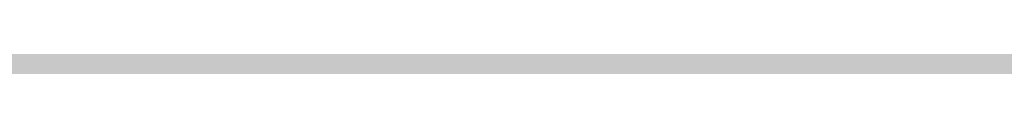
# Model space of a CAD drawing. Units: inches. Extents: x 2091 to 2899, y 967 to 2217.
# Tile 226 of 256: x 2203.4104 to 2203.7172, y 1152.2487 to 1152.2504. Entities that reach past the tile are written whole.
import ezdxf

# ---------------------------------------------------------------- set-up
doc = ezdxf.new("R2010")
doc.units = ezdxf.units.IN
doc.layers.add('A-WALL-PATT', color=141, linetype='Continuous', lineweight=13, true_color=0xadddf7)

msp = doc.modelspace()

# ---------------------------------------------------------------- hatches: boundary and pattern name
at = {"layer": 'A-WALL-PATT'}
h = msp.add_hatch(color=256, dxfattribs=at)
h.dxf.hatch_style = 1
h.paths.add_polyline_path([(2803.1436, 2050.91906), (2203.1436, 2050.91906), (2203.1436, 1090.91906), (2803.1436, 1090.91906)])
h.paths.add_polyline_path([(2635.79885, 1147.54046), (2674.52405, 1147.54046, 0.376086), (2678.52967, 1152.8802), (2678.52967, 1159.55647, 0.333335), (2674.52432, 1163.56185), (2674.52432, 1163.56185), (2674.52432, 1192.93439), (2635.80597, 1192.93439), (2597.08762, 1192.93439), (2597.08762, 1163.56185, 0.333335), (2593.08228, 1159.55647), (2593.08228, 1152.8802, 0.376086), (2597.08789, 1147.54046)], flags=0)
h.paths.add_polyline_path([(2436.01043, 1278.24078, 0.000483), (2435.95264, 1278.21503, -0.001328), (2435.93563, 1278.11169, -0.001711), (2436.11644, 1278.04076, 0.002185)], flags=0)
h.paths.add_polyline_path([(2794.1436, 1143.41906), (2794.1436, 1347.41906), (2543.37017, 1347.41906), (2543.37017, 1351.91906), (2794.1436, 1351.91906), (2794.1436, 1392.71355), (2793.9474, 1392.71355), (2793.9474, 1473.5369), (2794.1436, 1473.5369), (2794.1436, 1531.91906), (2650.1436, 1531.91906), (2650.1436, 1536.41906), (2794.1436, 1536.41906), (2794.1436, 1692.41906), (2609.37561, 1692.41906), (2609.37561, 1644.41906), (2604.87561, 1644.41906), (2604.87561, 1744.91906), (2609.37561, 1744.91906), (2609.37561, 1696.91906), (2794.1436, 1696.91906), (2794.1436, 1780.91906), (2609.6436, 1780.91906), (2493.87561, 1780.91906), (2493.87561, 1785.41906), (2609.6436, 1785.41906), (2794.1436, 1785.41906), (2794.1436, 1847.93882), (2793.95122, 1847.93882), (2793.95122, 1928.76217), (2794.1436, 1928.76217), (2794.1436, 1941.41906), (2614.1436, 1941.41906), (2614.1436, 1821.41906), (2609.6436, 1821.41906), (2609.6436, 1941.41906), (2392.1436, 1941.41906), (2392.1436, 1819.91906), (2387.6436, 1819.91906), (2387.6436, 1941.41906), (2212.1436, 1941.41906), (2212.1436, 1783.91906), (2392.1436, 1783.91906), (2392.1436, 1780.91906), (2212.1436, 1780.91906), (2212.1436, 1629.41906), (2387.6436, 1629.41906), (2387.6436, 1744.91906), (2392.1436, 1744.91906), (2392.1436, 1627.91906), (2317.1436, 1627.91906), (2317.1436, 1551.41906), (2317.1436, 1536.41906), (2459.38359, 1536.41906), (2459.38359, 1602.39648), (2463.88359, 1602.39648), (2463.88359, 1531.91906), (2456.6436, 1531.91906), (2456.6436, 1529.91906), (2452.1436, 1529.91906), (2452.1436, 1531.91906), (2312.6436, 1531.91906), (2312.6436, 1551.41906), (2306.1436, 1551.41906), (2306.1436, 1555.91906), (2308.1436, 1555.91906), (2308.1436, 1551.41906), (2312.6436, 1551.41906), (2312.6436, 1627.91906), (2212.1436, 1627.91906), (2212.1436, 1555.91906), (2270.1436, 1555.91906), (2270.1436, 1551.41906), (2212.1436, 1551.41906), (2212.1436, 1351.91906), (2272.1436, 1351.91906), (2272.1436, 1347.41906), (2212.1436, 1347.41906), (2212.1436, 1275.41906), (2308.1436, 1275.41906), (2308.1436, 1351.91906), (2452.1436, 1351.91906), (2452.1436, 1493.91906), (2456.6436, 1493.91906), (2456.6436, 1347.41906), (2312.6436, 1347.41906), (2312.6436, 1270.91906), (2212.1436, 1270.91906), (2212.1436, 1099.91906), (2281.23752, 1099.91906), (2282.87104, 1110.9138), (2282.00834, 1116.9966), (2278.55774, 1121.4204), (2268.20564, 1128.0562), (2272.08764, 1128.0562), (2273.81294, 1131.927), (2279.42034, 1134.6919), (2285.02784, 1135.2449), (2287.61584, 1137.4568), (2288.04714, 1138.0098), (2289.34114, 1140.7747), (2291.06654, 1139.6687), (2292.36054, 1135.2449), (2295.37984, 1136.9038), (2296.24254, 1135.7979), (2297.10524, 1133.033), (2300.12464, 1138.0098), (2303.14394, 1138.0098), (2304.43794, 1135.7979), (2303.14394, 1133.586), (2306.59464, 1134.6919), (2307.88874, 1133.033), (2310.90804, 1135.2449), (2313.92744, 1134.1389), (2315.62686, 1132.4271), (2308.32004, 1117.5496), (2290.20384, 1109.8079), (2288.90984, 1103.1721), (2289.27231, 1099.91906), (2434.91823, 1099.91906), (2431.59323, 1124.78806), (2429.93023, 1169.55306), (2430.92718, 1240.51969), (2435.65893, 1238.18613), (2437.13523, 1196.55406), (2438.79823, 1143.97306), (2442.67823, 1111.99806), (2446.55823, 1099.91906), (2794.1436, 1099.91906), (2794.1436, 1138.91906), (2548.03245, 1138.91906), (2548.03245, 1143.41906), (2548.03245, 1148.81906), (2546.66846, 1148.03156), (2528.68569, 1179.17862, 0.256256), (2512.03245, 1148.81906), (2512.03245, 1143.41906), (2512.03245, 1138.91906), (2507.53245, 1138.91906), (2507.53245, 1143.41906), (2507.53245, 1148.81906, 0.256256), (2490.8792, 1179.17862), (2472.89644, 1148.03156), (2471.53245, 1148.81906), (2471.53245, 1143.41906), (2467.03245, 1143.41906), (2467.03245, 1269.94579, 0.039061), (2460.90999, 1273.58006), (2467.03245, 1273.58006), (2467.03245, 1286.32536, 0.014511), (2465.21619, 1286.76191), (2467.03245, 1287.05258), (2467.03245, 1323.41906), (2471.53245, 1323.41906), (2471.53245, 1148.81906), (2489.53245, 1179.99597), (2490.89644, 1179.20847), (2490.8792, 1179.17862, -0.256256), (2507.53245, 1148.81906), (2507.53245, 1143.41906), (2512.03245, 1143.41906), (2512.03245, 1148.81906, -0.256256), (2528.68569, 1179.17862), (2528.66846, 1179.20847), (2530.03245, 1179.99597), (2548.03245, 1148.81906), (2548.03245, 1143.41906)], flags=16)
h.paths.add_polyline_path([(2607.76855, 1200.94508), (2607.76855, 1265.03063), (2597.08762, 1281.05201), (2619.78459, 1281.05201), (2627.79528, 1337.12686), (2635.79885, 1337.12686), (2643.81666, 1337.12686), (2651.82736, 1281.05201), (2674.52432, 1281.05201), (2663.8434, 1265.03063), (2663.8434, 1200.94508), (2635.80597, 1200.94508)], flags=0)
edge = h.paths.add_edge_path(flags=0)
edge.add_ellipse((13303.89622, 1272.99872), major_axis=(-10595.31304, 0), ratio=0.84230387009, start_angle=0.628237219, end_angle=0.6465541, ccw=False)
edge.add_ellipse((2711.70045, 1156.85268), major_axis=(2.21977, 0), ratio=0.8423039, start_angle=111.53524, end_angle=180.62824, ccw=False)
edge.add_ellipse((13303.15629, 1272.99872), major_axis=(-10593.02631, 0), ratio=0.84230386954, start_angle=0.528271472, end_angle=0.646554097, ccw=False)
edge.add_line((2710.7646, 1175.3333), (2710.12999, 1175.3333))
edge.add_ellipse((2710.12999, 1176.57978), major_axis=(1.47985, 0), ratio=0.8423039, start_angle=180, end_angle=270, ccw=False)
edge.add_line((2708.65014, 1176.57978), (2708.65014, 1200.78291))
edge.add_ellipse((2710.12999, 1200.78291), major_axis=(1.47985, 0), ratio=0.8423039, start_angle=90, end_angle=180, ccw=False)
edge.add_line((2710.12999, 1202.02939), (2710.46508, 1202.02939))
edge.add_ellipse((13303.15629, 1272.99872), major_axis=(-10593.02631, 0), ratio=0.84230386954, start_angle=-0.090229089, end_angle=0.383866779, ccw=False)
edge.add_ellipse((2710.12999, 1290.92703), major_axis=(-1.47985, 0), ratio=0.8423039, start_angle=0, end_angle=90, ccw=False)
edge.add_line((2708.65014, 1290.92703), (2708.65014, 1315.13017))
edge.add_ellipse((2710.12999, 1315.13017), major_axis=(-1.47985, 0), ratio=0.8423039, start_angle=-90, end_angle=0, ccw=False)
edge.add_line((2710.12999, 1316.37665), (2710.70631, 1316.37665))
edge.add_ellipse((3238.40172, 1296.28957), major_axis=(528.234, 0), ratio=0.84230387, start_angle=176.3495724, end_angle=177.8200497, ccw=False)
edge.add_ellipse((2775.06304, 1071.4507), major_axis=(313.30776, 0), ratio=0.84230387, start_angle=102.1259656, end_angle=103.780529, ccw=False)
edge.add_ellipse((2775.06304, 1078.3057), major_axis=(-305.30289, 0), ratio=0.84230387, start_angle=-79.790461, end_angle=-77.5553727, ccw=False)
edge.add_ellipse((2695.14177, 1541.97538), major_axis=(-250.96022, 0), ratio=0.84230387, start_angle=99.256566, end_angle=102.5549326)
edge.add_line((2741.41033, 1334.21426), (2747.13255, 1337.37848))
edge.add_ellipse((2747.53862, 1336.85748), major_axis=(-0.73992, 0), ratio=0.842304, start_angle=270, end_angle=307.93313, ccw=False)
edge.add_ellipse((2747.53862, 1336.85748), major_axis=(-0.73992, 0), ratio=0.842304, start_angle=232.06687, end_angle=270, ccw=False)
edge.add_line((2747.94469, 1337.37848), (2753.66691, 1334.21426))
edge.add_ellipse((2799.93547, 1541.97538), major_axis=(250.96022, 0), ratio=0.84230387, start_angle=257.4450674, end_angle=260.743434)
edge.add_ellipse((2720.01419, 1078.3057), major_axis=(305.30289, 0), ratio=0.84230387, start_angle=77.5553727, end_angle=79.790461, ccw=False)
edge.add_ellipse((2720.01419, 1071.4507), major_axis=(-313.30776, 0), ratio=0.84230387, start_angle=256.219471, end_angle=257.8740344, ccw=False)
edge.add_ellipse((2256.67551, 1296.28957), major_axis=(-528.234, 0), ratio=0.84230387, start_angle=182.1799503, end_angle=183.6504276, ccw=False)
edge.add_line((2784.37092, 1316.37665), (2784.94725, 1316.37665))
edge.add_ellipse((2784.94725, 1315.13017), major_axis=(1.47985, 0), ratio=0.8423039, start_angle=0, end_angle=90, ccw=False)
edge.add_line((2786.42709, 1315.13017), (2786.42709, 1290.92703))
edge.add_ellipse((2784.94725, 1290.92703), major_axis=(1.47985, 0), ratio=0.8423039, start_angle=270, end_angle=360, ccw=False)
edge.add_ellipse((-7808.07906, 1272.99872), major_axis=(10593.02631, 0), ratio=0.84230386954, start_angle=-0.383866779, end_angle=0.090229089, ccw=False)
edge.add_line((2784.61216, 1202.02939), (2784.94725, 1202.02939))
edge.add_ellipse((2784.94725, 1200.78291), major_axis=(1.47985, 0), ratio=0.8423039, start_angle=0, end_angle=90, ccw=False)
edge.add_line((2786.42709, 1200.78291), (2786.42709, 1176.57978))
edge.add_ellipse((2784.94725, 1176.57978), major_axis=(-1.47985, 0), ratio=0.8423039, start_angle=90, end_angle=180, ccw=False)
edge.add_line((2784.94725, 1175.3333), (2784.31264, 1175.3333))
edge.add_ellipse((-7808.07906, 1272.99872), major_axis=(10593.02631, 0), ratio=0.84230386954, start_angle=-0.618643196, end_angle=-0.528271472, ccw=False)
edge.add_ellipse((2783.37678, 1156.85268), major_axis=(-2.21977, 0), ratio=0.8423039, start_angle=179.37176, end_angle=248.46476, ccw=False)
edge.add_ellipse((-7808.81898, 1272.99872), major_axis=(-10595.31304, 0), ratio=0.84230386576, start_angle=179.353445923, end_angle=179.371762803, ccw=False)
edge.add_ellipse((2780.2973, 1153.50079), major_axis=(-5.24643, 0), ratio=0.8423039, start_angle=90, end_angle=179.35345, ccw=False)
edge.add_line((2780.2973, 1149.08171), (2714.77993, 1149.08171))
edge.add_ellipse((2714.77993, 1153.50079), major_axis=(5.24643, 0), ratio=0.8423039, start_angle=180.64655, end_angle=270, ccw=False)
edge = h.paths.add_edge_path(flags=0)
edge.add_line((2718.18737, 1151.00783), (2718.18737, 1170.47236))
edge.add_ellipse((2721.14706, 1170.47236), major_axis=(-2.95969, 0), ratio=0.8423039, start_angle=-90, end_angle=0, ccw=False)
edge.add_line((2721.14706, 1172.96532), (2773.93017, 1172.96532))
edge.add_ellipse((2773.93017, 1170.47236), major_axis=(-2.95969, 0), ratio=0.8423039, start_angle=180, end_angle=270, ccw=False)
edge.add_line((2776.88987, 1170.47236), (2776.88987, 1151.00783))
edge.add_line((2776.88987, 1151.00783), (2718.18737, 1151.00783))
edge = h.paths.add_edge_path(flags=0)
edge.add_line((2718.18737, 1180.23415), (2718.18737, 1199.05783))
edge.add_ellipse((2747.53862, 1320.39864), major_axis=(147.01792, 0), ratio=0.84230387, start_angle=256.4018653, end_angle=283.5981347)
edge.add_line((2776.88987, 1199.05783), (2776.88987, 1180.23415))
edge.add_ellipse((2747.53862, 1301.57496), major_axis=(147.01792, 0), ratio=0.84230387, start_angle=256.4018653, end_angle=283.5981347, ccw=False)
edge = h.paths.add_edge_path(flags=0)
edge.add_ellipse((13303.15629, 1272.99872), major_axis=(-10591.54646, 0), ratio=0.84230386955, start_angle=0.055594314, end_angle=0.377764194, ccw=False)
edge.add_line((2711.61686, 1262.72171), (2715.66741, 1249.4954))
edge.add_ellipse((6413.89196, 1241.69192), major_axis=(-3698.23616, 0), ratio=0.8423038695, start_angle=-0.12089737, end_angle=0.36407635)
edge.add_line((2715.76104, 1218.19245), (2711.93431, 1203.16736))
edge = h.paths.add_edge_path(flags=0)
edge.add_line((2718.18737, 1251.07457), (2716.00249, 1267.45044))
edge.add_ellipse((2742.15117, 1202.18954), major_axis=(81.77258, 0), ratio=0.84230387, start_angle=94.277421, end_angle=111.8349538, ccw=False)
edge.add_line((2737.00975, 1270.93063), (2758.06748, 1270.93063))
edge.add_ellipse((2752.92606, 1202.18954), major_axis=(81.77258, 0), ratio=0.84230387, start_angle=68.1650462, end_angle=85.722579, ccw=False)
edge.add_line((2779.07475, 1267.45044), (2776.88987, 1251.07457))
edge.add_ellipse((2750.33806, 1187.88536), major_axis=(79.57966, 0), ratio=0.84230387, start_angle=67.2080851, end_angle=85.1299304)
edge.add_line((2756.03466, 1254.74366), (2739.04258, 1254.74366))
edge.add_ellipse((2744.73917, 1187.88536), major_axis=(79.57966, 0), ratio=0.84230387, start_angle=94.8700696, end_angle=112.7919149)
edge = h.paths.add_edge_path(flags=0)
edge.add_line((2783.14293, 1203.16736), (2779.31619, 1218.19245))
edge.add_ellipse((-918.81473, 1241.69192), major_axis=(3698.23616, 0), ratio=0.8423038695, start_angle=-0.36407635, end_angle=0.12089737)
edge.add_line((2779.40983, 1249.4954), (2783.46037, 1262.72171))
edge.add_ellipse((-7808.07906, 1272.99872), major_axis=(-10591.54646, 0), ratio=0.84230386954, start_angle=179.622235806, end_angle=179.944405687, ccw=False)
edge = h.paths.add_edge_path(flags=0)
edge.add_ellipse((2734.20089, 1286.69044), major_axis=(-0.35661, 6.34008), ratio=0.6038336, start_angle=89.002014, end_angle=253.657408, ccw=False)
edge.add_line((2730.369, 1286.54181), (2730.369, 1301.35198))
edge.add_line((2730.369, 1301.35198), (2735.91331, 1305.2148))
edge.add_ellipse((2736.38492, 1304.73456), major_axis=(0.73992, 0), ratio=0.842304, start_angle=90, end_angle=134.48021, ccw=False)
edge.add_line((2736.38492, 1305.3578), (2738.03278, 1305.3578))
edge.add_line((2738.03278, 1305.3578), (2738.03278, 1307.70793))
edge.add_ellipse((2794.20164, 1307.70793), major_axis=(56.16886, 0), ratio=0.84230387, start_angle=150.56143, end_angle=180, ccw=False)
edge.add_ellipse((2700.87559, 1307.70793), major_axis=(-56.16886, 0), ratio=0.84230387, start_angle=180, end_angle=209.43857, ccw=False)
edge.add_line((2757.04445, 1307.70793), (2757.04445, 1305.3578))
edge.add_line((2757.04445, 1305.3578), (2758.69232, 1305.3578))
edge.add_ellipse((2758.69232, 1304.73456), major_axis=(-0.73992, 0), ratio=0.842304, start_angle=225.51979, end_angle=270, ccw=False)
edge.add_line((2759.16392, 1305.2148), (2764.70823, 1301.35198))
edge.add_line((2764.70823, 1301.35198), (2764.70823, 1286.54181))
edge.add_ellipse((2760.87634, 1286.69044), major_axis=(0.35661, 6.34008), ratio=0.6038336, start_angle=106.342592, end_angle=270.997986, ccw=False)
edge.add_line((2757.04445, 1285.79709), (2757.04445, 1307.70793))
edge.add_ellipse((2700.87559, 1307.70793), major_axis=(-56.16886, 0), ratio=0.84230387, start_angle=180, end_angle=209.43857)
edge.add_ellipse((2794.20164, 1307.70793), major_axis=(56.16886, 0), ratio=0.84230387, start_angle=150.56143, end_angle=180)
edge.add_line((2738.03278, 1307.70793), (2738.03278, 1285.79709))
h.paths.add_polyline_path([(2417.81227, 1104.4497), (2413.49227, 1102.5297), (2410.61227, 1103.9697), (2409.17227, 1106.3697), (2407.25227, 1107.3297), (2406.29227, 1109.7297), (2405.33227, 1114.0497), (2405.33227, 1117.8897), (2406.29227, 1120.1297), (2407.25227, 1119.8097), (2408.84832, 1118.32766), (2410.17395, 1119.42417), (2410.21127, 1120.4057), (2411.04073, 1121.41905), (2410.69927, 1119.8587), (2410.17395, 1119.42417), (2410.08845, 1117.17611), (2411.13284, 1116.20632), (2413.97227, 1119.3297), (2416.85227, 1120.7697), (2416.86972, 1120.79878), (2417.03507, 1119.40512), (2417.89621, 1118.14338), (2418.29227, 1118.3697), (2419.54445, 1120.03927), (2419.36092, 1118.38749), (2419.03211, 1119.35615), (2418.39894, 1118.51193), (2419.25227, 1114.5297), (2418.79409, 1107.19879)], flags=0)
h.paths.add_polyline_path([(2508.87017, 1347.41906), (2508.37017, 1347.41906), (2508.37017, 1351.91906), (2508.87017, 1351.91906)], flags=0)
h.paths.add_polyline_path([(2473.37017, 1347.41906), (2472.37017, 1347.41906), (2467.87017, 1347.41906), (2467.87017, 1455.41906), (2472.37017, 1455.41906), (2472.37017, 1352.41906), (2473.37017, 1352.41906)], flags=0)
h.paths.add_polyline_path([(2352.10624, 1217.4462), (2349.22624, 1218.8862), (2347.78624, 1221.2862), (2345.86624, 1222.2462), (2344.90624, 1224.6462), (2343.94624, 1228.9662), (2343.94624, 1232.8062), (2344.90624, 1235.0462), (2345.86624, 1234.7262), (2347.46229, 1233.24415), (2348.78792, 1234.34066), (2348.82524, 1235.3222), (2349.6547, 1236.33555), (2349.31324, 1234.7752), (2348.78792, 1234.34066), (2348.70242, 1232.0926), (2349.74681, 1231.12282), (2352.58624, 1234.2462), (2355.46624, 1235.6862), (2355.48369, 1235.71528), (2355.64904, 1234.32161), (2356.51018, 1233.05988), (2356.90624, 1233.2862), (2358.15842, 1234.95576), (2357.97489, 1233.30398), (2357.64608, 1234.27264), (2357.01291, 1233.42842), (2357.86624, 1229.4462), (2357.40806, 1222.11529), (2356.42624, 1219.3662)], flags=0)
h.paths.add_polyline_path([(2348.2968, 1112.22442), (2347.0138, 1112.31042), (2345.5298, 1114.12742), (2345.7318, 1115.85842), (2346.8118, 1116.98242), (2346.8118, 1114.64642), (2345.8668, 1114.21442), (2346.8798, 1114.30042)], flags=0)
h.paths.add_polyline_path([(2347.0138, 1110.92642), (2346.2718, 1110.49342), (2346.6098, 1111.18642)], flags=0)
h.paths.add_polyline_path([(2345.8668, 1118.19442), (2345.5298, 1117.32942), (2343.7078, 1118.02142), (2344.3828, 1118.62642)], flags=0)
h.paths.add_polyline_path([(2346.6768, 1109.28242), (2346.0698, 1108.07142), (2345.8668, 1110.06142)], flags=0)
h.paths.add_polyline_path([(2345.0568, 1119.75142), (2343.6398, 1119.75142), (2343.9778, 1121.13542)], flags=0)
h.paths.add_polyline_path([(2345.2598, 1116.55042), (2345.1248, 1115.85842), (2344.9218, 1115.68542), (2344.7198, 1116.37742)], flags=0)
h.paths.add_polyline_path([(2345.6648, 1112.31042), (2345.4618, 1111.53242), (2344.0448, 1111.96442), (2344.6518, 1112.57042)], flags=0)
h.paths.add_polyline_path([(2345.1918, 1113.34942), (2344.4498, 1113.86842), (2344.7198, 1114.38742)], flags=0)
h.paths.add_polyline_path([(2344.6518, 1116.80942), (2344.1798, 1115.68542), (2344.6518, 1115.33942), (2343.9098, 1114.90642), (2343.0328, 1115.94442), (2343.6398, 1116.46342)], flags=0)
h.paths.add_polyline_path([(2345.8668, 1106.68642), (2344.9898, 1105.56242), (2344.5168, 1106.60042)], flags=0)
h.paths.add_polyline_path([(2344.8548, 1110.06142), (2344.5168, 1109.28242), (2344.1128, 1109.71542)], flags=0)
h.paths.add_polyline_path([(2344.0448, 1113.52242), (2343.4378, 1113.08942), (2342.7628, 1113.95442)], flags=0)
h.paths.add_polyline_path([(2344.3148, 1111.01242), (2342.9648, 1110.32042), (2342.9648, 1111.09942)], flags=0)
h.paths.add_polyline_path([(2345.1248, 1104.69742), (2344.5848, 1103.74542), (2344.4498, 1104.26442)], flags=0)
h.paths.add_polyline_path([(2342.8298, 1121.22242), (2341.7498, 1120.53042), (2340.5358, 1121.04942), (2340.1308, 1121.82842), (2340.6708, 1122.95242), (2341.1428, 1121.82842), (2341.6148, 1122.00142)], flags=0)
h.paths.add_polyline_path([(2342.9648, 1119.75142), (2343.0328, 1118.45342), (2342.0878, 1118.02142), (2342.0198, 1119.49142)], flags=0)
h.paths.add_polyline_path([(2342.6948, 1116.89642), (2341.9528, 1116.63642), (2342.0198, 1117.32942)], flags=0)
h.paths.add_polyline_path([(2343.0328, 1112.22442), (2342.0198, 1111.79142), (2341.5478, 1112.22442), (2342.3578, 1113.34942)], flags=0)
h.paths.add_polyline_path([(2343.7748, 1104.43742), (2342.6278, 1102.88042), (2342.6948, 1104.61042), (2343.4378, 1105.12942)], flags=0)
h.paths.add_polyline_path([(2342.0198, 1115.07942), (2340.8058, 1115.51242), (2340.9408, 1116.37742)], flags=0)
h.paths.add_polyline_path([(2341.4808, 1120.09742), (2341.4808, 1119.40542), (2341.0758, 1119.57842), (2341.1428, 1120.09742)], flags=0)
h.paths.add_polyline_path([(2341.8178, 1114.47342), (2340.9408, 1113.08942), (2340.8058, 1114.56042)], flags=0)
h.paths.add_polyline_path([(2341.1428, 1118.54042), (2340.9408, 1116.98242), (2339.0508, 1117.67542), (2339.0508, 1118.62642)], flags=0)
h.paths.add_polyline_path([(2342.6948, 1101.66842), (2341.9528, 1101.84142), (2342.5598, 1102.36142)], flags=0)
h.paths.add_polyline_path([(2340.3328, 1119.66542), (2338.4438, 1119.57842), (2337.9038, 1120.35742), (2339.6578, 1120.61642)], flags=0)
h.paths.add_polyline_path([(2340.3328, 1115.33942), (2340.0628, 1113.69542), (2339.3878, 1115.33942)], flags=0)
h.paths.add_polyline_path([(2341.8178, 1103.83142), (2341.5478, 1102.88042), (2341.1428, 1103.65842)], flags=0)
h.paths.add_polyline_path([(2339.0508, 1122.86642), (2337.2958, 1121.82842), (2337.0938, 1123.12542), (2337.7688, 1123.81842)], flags=0)
h.paths.add_polyline_path([(2339.1178, 1121.74142), (2338.8478, 1121.22242), (2338.1738, 1121.04942), (2338.3758, 1121.56842)], flags=0)
h.paths.add_polyline_path([(2339.1858, 1119.31942), (2338.6458, 1118.71342), (2338.2408, 1118.10742), (2338.2408, 1118.88642)], flags=0)
h.paths.add_polyline_path([(2341.1428, 1101.92842), (2340.6028, 1101.23642), (2340.0628, 1101.84142), (2340.6028, 1102.36142)], flags=0)
h.paths.add_polyline_path([(2337.6338, 1117.76142), (2336.6208, 1118.28042), (2337.2958, 1118.97242)], flags=0)
h.paths.add_polyline_path([(2336.8238, 1119.57842), (2334.7988, 1118.97242), (2335.2038, 1120.35742), (2336.5538, 1120.87642)], flags=0)
h.paths.add_polyline_path([(2339.1178, 1100.45742), (2337.3638, 1100.54342), (2336.7558, 1101.23642)], flags=0)
h.paths.add_polyline_path([(2336.3508, 1122.43342), (2336.0138, 1121.91442), (2334.9338, 1122.43342), (2334.5288, 1123.47142), (2335.7438, 1122.77942)], flags=0)
h.paths.add_polyline_path([(2334.7318, 1120.87642), (2334.2588, 1120.35742), (2334.0568, 1120.78942), (2334.5968, 1121.30842)], flags=0)
h.paths.add_polyline_path([(2334.4618, 1122.17442), (2332.5718, 1121.30842), (2331.3568, 1122.17442), (2332.0998, 1122.86642)], flags=0)
h.paths.add_polyline_path([(2334.2588, 1118.54042), (2333.3818, 1118.45342), (2333.6518, 1119.31942)], flags=0)
h.paths.add_polyline_path([(2335.5418, 1102.27442), (2334.1918, 1102.62042), (2335.2718, 1103.31242)], flags=0)
h.paths.add_polyline_path([(2332.7068, 1119.66542), (2331.6948, 1120.44342), (2332.5048, 1120.78942)], flags=0)
h.paths.add_polyline_path([(2334.7318, 1101.14942), (2333.5168, 1101.58242), (2333.9888, 1101.75542)], flags=0)
h.paths.add_polyline_path([(2332.6398, 1116.63642), (2331.0868, 1116.29042), (2331.9648, 1118.19442)], flags=0)
h.paths.add_polyline_path([(2330.7498, 1121.56842), (2330.2768, 1120.27042), (2328.5228, 1119.31942), (2328.9948, 1121.04942)], flags=0)
h.paths.add_polyline_path([(2330.7498, 1118.62642), (2330.0078, 1117.50242), (2329.8728, 1118.02142)], flags=0)
h.paths.add_polyline_path([(2332.0998, 1102.36142), (2330.5468, 1102.01442), (2331.6948, 1102.96642)], flags=0)
h.paths.add_polyline_path([(2329.5348, 1113.60842), (2329.0628, 1112.31042), (2328.5898, 1113.34942)], flags=0)
h.paths.add_polyline_path([(2328.3878, 1117.84842), (2327.5098, 1116.55042), (2327.1728, 1117.76142)], flags=0)
h.paths.add_polyline_path([(2329.7378, 1106.51342), (2329.5348, 1105.30242), (2328.2528, 1106.08142)], flags=0)
h.paths.add_polyline_path([(2328.6578, 1114.38742), (2328.0498, 1114.12742), (2328.3198, 1114.90642)], flags=0)
h.paths.add_polyline_path([(2328.3198, 1112.22442), (2327.1058, 1112.13742), (2326.7008, 1112.65642)], flags=0)
h.paths.add_polyline_path([(2326.9028, 1115.25242), (2326.7008, 1114.12742), (2325.2158, 1113.60842), (2326.0928, 1115.33942)], flags=0)
h.paths.add_polyline_path([(2326.6328, 1108.33042), (2326.0928, 1107.37942), (2325.8908, 1108.50342), (2326.4978, 1109.10942)], flags=0)
h.paths.add_polyline_path([(2615.1436, 1531.91906), (2609.6436, 1531.91906), (2609.6436, 1620.41906), (2614.1436, 1620.41906), (2614.1436, 1536.41906), (2615.1436, 1536.41906)], flags=0)
h.paths.add_polyline_path([(2545.1436, 1563.41906), (2464.1436, 1563.41906), (2464.1436, 1632.41906), (2509.1436, 1632.41906), (2509.1436, 1627.91906), (2509.1436, 1603.91906), (2468.6436, 1603.91906), (2468.6436, 1567.91906), (2540.6436, 1567.91906), (2540.6436, 1591.91906), (2545.1436, 1591.91906)], flags=0)
h.paths.add_polyline_path([(2388.96905, 1549.98573), (2357.43418, 1549.98573), (2357.43418, 1623.36078), (2399.36278, 1623.36078), (2435.68947, 1623.36078), (2435.59255, 1602.55927), (2435.59255, 1602.39648), (2388.96905, 1602.39648)], flags=0)
h.paths.add_polyline_path([(2388.88063, 1555.80915), (2374.90443, 1555.80915), (2374.90443, 1600.57156), (2374.90443, 1615.45765), (2406.35088, 1615.45765), (2406.35088, 1618.93943), (2412.17429, 1615.45765), (2406.35088, 1611.97586), (2406.35088, 1615.45765), (2388.88063, 1615.45765)], flags=0)
h.paths.add_polyline_path([(2568.87561, 1644.41906), (2453.37561, 1644.41906), (2453.37561, 1785.41906), (2457.87561, 1785.41906), (2457.87561, 1648.91906), (2568.87561, 1648.91906)], flags=0)
h.paths.add_polyline_path([(2212.1436, 1945.91906), (2212.1436, 2041.91906), (2794.1436, 2041.91906), (2794.1436, 1945.91906)], flags=16)
h.paths.add_polyline_path([(2271.08273, 1964.31724), (2776.85297, 1964.31724), (2776.85297, 2037.16962), (2271.08273, 2037.16962)], flags=8)
h.paths.add_polyline_path([(2380.64929, 1536.82414), (2461.04081, 1536.82414), (2461.04081, 1554.65259), (2380.64929, 1554.65259)], flags=8)
h.paths.add_polyline_path([(2240.75571, 1609.72545), (2309.18583, 1609.72545), (2309.18583, 1617.6982), (2240.75571, 1617.6982)], flags=8)
h.paths.add_polyline_path([(2212.67726, 1313.5041), (2282.59152, 1313.5041), (2282.59152, 1322.74524), (2212.67726, 1322.74524)], flags=8)
h.paths.add_polyline_path([(2457.11198, 1114.77857), (2558.48158, 1114.77857), (2558.48158, 1142.21968), (2457.11198, 1142.21968)], flags=8)
h.paths.add_polyline_path([(2473.44234, 1273.01007), (2604.64123, 1273.01007), (2604.64123, 1318.34693), (2473.44234, 1318.34693)], flags=8)
h.paths.add_polyline_path([(2638.8763, 1626.97743), (2684.25037, 1627.97674), (2684.03848, 1637.59749), (2638.66442, 1636.59819)], flags=8)
h.paths.add_polyline_path([(2537.59055, 1453.79345), (2628.38955, 1453.79345), (2628.38955, 1475.34481), (2537.59055, 1475.34481)], flags=8)
h.paths.add_polyline_path([(2504.13764, 1714.6324), (2554.64719, 1714.6324), (2554.64719, 1730.23771), (2504.13764, 1730.23771)], flags=8)
h.paths.add_polyline_path([(2487.50118, 1575.65187), (2535.09712, 1575.65187), (2535.09712, 1598.37765), (2487.50118, 1598.37765)], flags=8)
h.paths.add_polyline_path([(2709.0994, 1735.71028), (2740.0166, 1735.71028), (2740.0166, 1749.93764), (2709.0994, 1749.93764)], flags=8)
h.paths.add_polyline_path([(2442.43842, 1792.17166), (2564.72884, 1792.17166), (2564.72884, 1842.00016), (2442.43842, 1842.00016)], flags=8)
h.paths.add_polyline_path([(2655.8158, 1809.64408), (2789.52014, 1806.6938), (2790.08498, 1832.29164), (2656.38064, 1835.24192)], flags=8)
h.paths.add_polyline_path([(2234.8427, 1797.72014), (2368.59285, 1794.76885), (2369.16072, 1820.50413), (2235.41056, 1823.45542)], flags=8)
h.paths.add_polyline_path([(2245.13847, 1644.00633), (2398.42773, 1640.6239), (2398.99484, 1666.32482), (2245.70557, 1669.70725)], flags=8)
h.paths.add_polyline_path([(2306.14285, 1431.16852), (2413.76831, 1428.79369), (2414.33315, 1454.39153), (2306.70768, 1456.76636)], flags=8)
h.paths.add_polyline_path([(2306.83458, 1458.23314), (2393.38048, 1456.32345), (2393.93281, 1481.35436), (2307.38691, 1483.26405)], flags=8)

doc.saveas('drawing.dxf')
